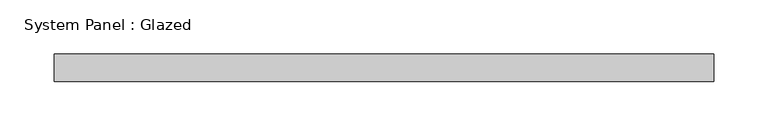
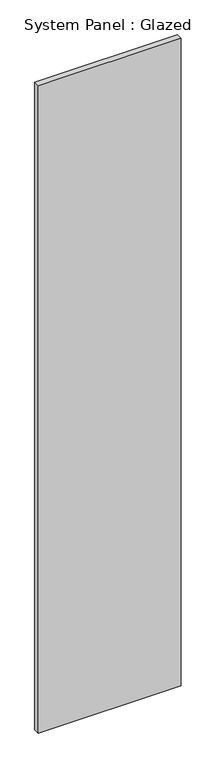
"""IFC4 building model written with IfcOpenShell, lengths in millimetres: plate geometry, System Panel : Glazed."""

from ifc_helpers import new_model, si_unit, origin, origin_with_axes, place, context, project, spatial, polyline, outline, extrude, source, transform, mapped, element, save


def system_panel_glazed_7c349084(model_context):
    return source(origin(), model_context, "Body", "SweptSolid", [
        extrude(outline(polyline([(304.8, 19.05), (-304.8, 19.05), (-304.8, 44.45), (304.8, 44.45), (304.8, 19.05)])), origin_with_axes(), (0.0, 0.0, 1.0), 2921.0),
    ])


if __name__ == "__main__":
    model = new_model("IFC4")
    model_context = context("Model", 3, world=origin())
    ifc_project = project(units=[si_unit("LENGTHUNIT", "METRE", prefix="MILLI")], contexts=[model_context])
    site = spatial("IfcSite", under=ifc_project)
    building = spatial("IfcBuilding", under=site)
    placement = place(None, origin())
    system_panel_glazed_shape = system_panel_glazed_7c349084(model_context)
    element("IfcPlate", 1, ObjectType="System Panel : Glazed", at=placement, inside=building, context=model_context, shape_type="MappedRepresentation", body=[
        mapped(system_panel_glazed_shape, transform((0.0, 0.0, 0.0), x_axis=(1.0, 0.0, 0.0), y_axis=(0.0, 1.0, 0.0), z_axis=(0.0, 0.0, 1.0))),
    ])
    save(model, "model.ifc")

# Revit data of these elements
# Type "System Panel : Glazed"
#   Construction Type Id = "GSP4R"
#   Analytic Construction = "1/8 in Pilkington single glazing"
#   Visual Light Transmittance = 0.9
#   Solar Heat Gain Coefficient = 0.86
#   Heat Transfer Coefficient (U) = 1.18115 BTU/(h·ft²·°F)
#   Define Thermal Properties by = 1
# Element 1 (IfcPlate, "System Panel : Glazed")
#   Materials on its faces: "Glass"
# Materials
#   "Glass": class "Glass", colour RGB 0 128 192, transparency 0.75, Description = "Soda Lime Glass", Cost = 0
